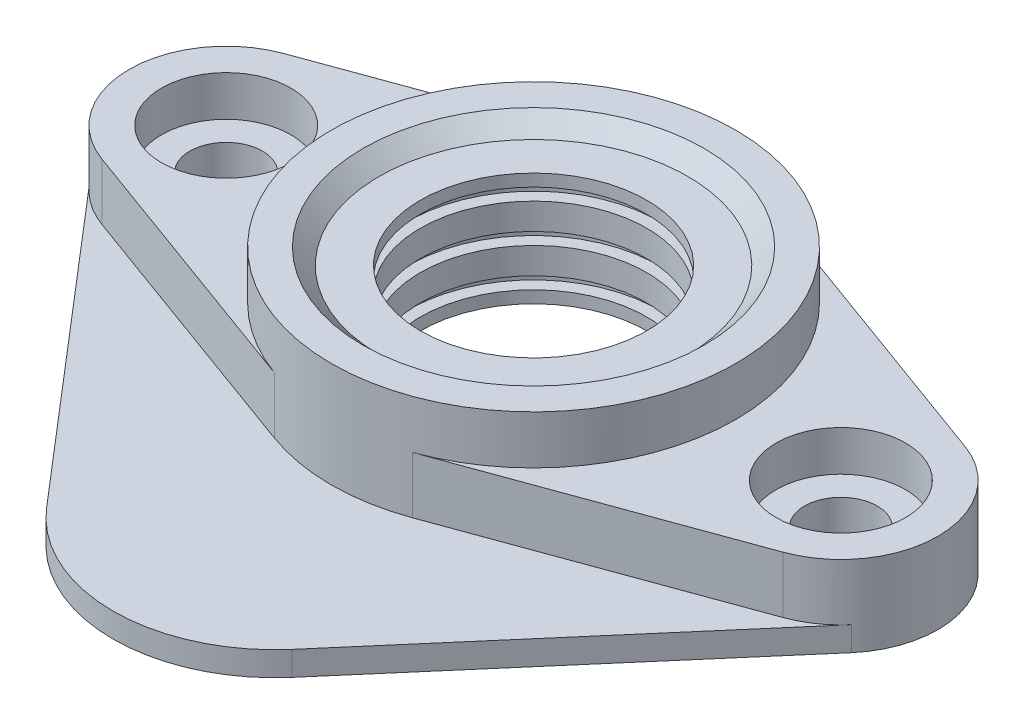
ISO-10303-21;
HEADER;
FILE_DESCRIPTION(('STEP AP214'),'2;1');
FILE_NAME('part.step','',(''),(''),'','','');
FILE_SCHEMA(('AUTOMOTIVE_DESIGN { 1 0 10303 214 1 1 1 1 }'));
ENDSEC;
DATA;
#1=APPLICATION_CONTEXT('core data for automotive mechanical design processes');
#2=APPLICATION_PROTOCOL_DEFINITION('international standard','automotive_design',2000,#1);
#3=PRODUCT_CONTEXT('',#1,'mechanical');
#4=PRODUCT('Part','Part','',(#3));
#5=PRODUCT_RELATED_PRODUCT_CATEGORY('part','',(#4));
#6=PRODUCT_DEFINITION_FORMATION('','',#4);
#7=PRODUCT_DEFINITION_CONTEXT('part definition',#1,'design');
#8=PRODUCT_DEFINITION('design','',#6,#7);
#9=PRODUCT_DEFINITION_SHAPE('','',#8);
#10=(LENGTH_UNIT() NAMED_UNIT(*) SI_UNIT(.MILLI.,.METRE.));
#11=(NAMED_UNIT(*) PLANE_ANGLE_UNIT() SI_UNIT($,.RADIAN.));
#12=(NAMED_UNIT(*) SI_UNIT($,.STERADIAN.) SOLID_ANGLE_UNIT());
#13=UNCERTAINTY_MEASURE_WITH_UNIT(LENGTH_MEASURE(1.E-05),#10,'distance_accuracy_value','');
#14=(GEOMETRIC_REPRESENTATION_CONTEXT(3) GLOBAL_UNCERTAINTY_ASSIGNED_CONTEXT((#13)) GLOBAL_UNIT_ASSIGNED_CONTEXT((#10,
#11,#12)) REPRESENTATION_CONTEXT('',''));
#15=CARTESIAN_POINT('',(0.,0.,0.));
#16=DIRECTION('',(0.,0.,1.));
#17=DIRECTION('',(1.,0.,0.));
#18=AXIS2_PLACEMENT_3D('',#15,#16,#17);
#19=CARTESIAN_POINT('',(-38.,3.,0.));
#20=DIRECTION('',(0.,1.,0.));
#21=DIRECTION('',(0.,0.,1.));
#22=AXIS2_PLACEMENT_3D('',#19,#20,#21);
#23=PLANE('',#22);
#24=DIRECTION('',(0.939661635334586,0.,-0.342105263157895));
#25=VECTOR('',#24,1.);
#26=CARTESIAN_POINT('',(8.55263157894737,3.,23.4915408833646));
#27=LINE('',#26,#25);
#28=CARTESIAN_POINT('',(8.55263157894736,3.,23.4915408833646));
#29=VERTEX_POINT('',#28);
#30=CARTESIAN_POINT('',(42.1052631578947,3.,11.275939624015));
#31=VERTEX_POINT('',#30);
#32=EDGE_CURVE('E69',#29,#31,#27,.T.);
#33=ORIENTED_EDGE('',*,*,#32,.F.);
#34=CARTESIAN_POINT('',(0.,3.,0.));
#35=DIRECTION('',(0.,1.,0.));
#36=DIRECTION('',(0.,0.,1.));
#37=AXIS2_PLACEMENT_3D('',#34,#35,#36);
#38=CIRCLE('',#37,25.);
#39=CARTESIAN_POINT('',(-8.55263157894736,3.,23.4915408833646));
#40=VERTEX_POINT('',#39);
#41=EDGE_CURVE('E264',#40,#29,#38,.T.);
#42=ORIENTED_EDGE('',*,*,#41,.F.);
#43=DIRECTION('',(0.939661635334586,0.,0.342105263157895));
#44=VECTOR('',#43,1.);
#45=CARTESIAN_POINT('',(-8.55263157894737,3.,23.4915408833646));
#46=LINE('',#45,#44);
#47=CARTESIAN_POINT('',(-42.1052631578947,3.,11.275939624015));
#48=VERTEX_POINT('',#47);
#49=EDGE_CURVE('E175',#48,#40,#46,.T.);
#50=ORIENTED_EDGE('',*,*,#49,.F.);
#51=CARTESIAN_POINT('',(-38.,3.,0.));
#52=DIRECTION('',(0.,1.,0.));
#53=DIRECTION('',(0.,0.,1.));
#54=AXIS2_PLACEMENT_3D('',#51,#52,#53);
#55=CIRCLE('',#54,12.);
#56=CARTESIAN_POINT('',(-47.1068684896246,3.,7.81440633142926));
#57=VERTEX_POINT('',#56);
#58=EDGE_CURVE('E11',#57,#48,#55,.T.);
#59=ORIENTED_EDGE('',*,*,#58,.F.);
#60=DIRECTION('',(0.651200527619105,0.,0.75890570746872));
#61=VECTOR('',#60,1.);
#62=CARTESIAN_POINT('',(-47.1068684896246,3.,7.81440633142926));
#63=LINE('',#62,#61);
#64=CARTESIAN_POINT('',(-15.1781141493744,3.,45.0240105523821));
#65=VERTEX_POINT('',#64);
#66=EDGE_CURVE('E192',#57,#65,#63,.T.);
#67=ORIENTED_EDGE('',*,*,#66,.T.);
#68=CARTESIAN_POINT('',(0.,3.,32.));
#69=DIRECTION('',(0.,1.,0.));
#70=DIRECTION('',(0.,0.,1.));
#71=AXIS2_PLACEMENT_3D('',#68,#69,#70);
#72=CIRCLE('',#71,20.);
#73=CARTESIAN_POINT('',(15.1781141493744,3.,45.0240105523821));
#74=VERTEX_POINT('',#73);
#75=EDGE_CURVE('E193',#65,#74,#72,.T.);
#76=ORIENTED_EDGE('',*,*,#75,.T.);
#77=DIRECTION('',(0.651200527619105,0.,-0.75890570746872));
#78=VECTOR('',#77,1.);
#79=CARTESIAN_POINT('',(47.1068684896246,3.,7.81440633142926));
#80=LINE('',#79,#78);
#81=CARTESIAN_POINT('',(47.1068684896246,3.,7.81440633142926));
#82=VERTEX_POINT('',#81);
#83=EDGE_CURVE('E197',#74,#82,#80,.T.);
#84=ORIENTED_EDGE('',*,*,#83,.T.);
#85=CARTESIAN_POINT('',(38.,3.,0.));
#86=DIRECTION('',(0.,1.,0.));
#87=DIRECTION('',(0.,0.,1.));
#88=AXIS2_PLACEMENT_3D('',#85,#86,#87);
#89=CIRCLE('',#88,12.);
#90=EDGE_CURVE('E61',#31,#82,#89,.T.);
#91=ORIENTED_EDGE('',*,*,#90,.F.);
#92=EDGE_LOOP('',(#33,#42,#50,#59,#67,#76,#84,#91));
#93=FACE_BOUND('',#92,.T.);
#94=ADVANCED_FACE('F50',(#93),#23,.T.);
#95=CARTESIAN_POINT('',(-38.,3.,0.));
#96=DIRECTION('',(0.,-1.,0.));
#97=DIRECTION('',(0.,0.,-1.));
#98=AXIS2_PLACEMENT_3D('',#95,#96,#97);
#99=CYLINDRICAL_SURFACE('',#98,12.);
#100=CARTESIAN_POINT('',(-38.,0.,0.));
#101=DIRECTION('',(0.,1.,0.));
#102=DIRECTION('',(0.,0.,1.));
#103=AXIS2_PLACEMENT_3D('',#100,#101,#102);
#104=CIRCLE('',#103,12.);
#105=CARTESIAN_POINT('',(-42.1052631578947,0.,-11.275939624015));
#106=VERTEX_POINT('',#105);
#107=CARTESIAN_POINT('',(-47.1068684896246,0.,7.81440633142926));
#108=VERTEX_POINT('',#107);
#109=EDGE_CURVE('E191',#106,#108,#104,.T.);
#110=ORIENTED_EDGE('',*,*,#109,.T.);
#111=DIRECTION('',(0.,-1.,0.));
#112=VECTOR('',#111,1.);
#113=CARTESIAN_POINT('',(-47.1068684896246,3.,7.81440633142926));
#114=LINE('',#113,#112);
#115=EDGE_CURVE('E51',#57,#108,#114,.T.);
#116=ORIENTED_EDGE('',*,*,#115,.F.);
#117=ORIENTED_EDGE('',*,*,#58,.T.);
#118=DIRECTION('',(0.,-1.,0.));
#119=VECTOR('',#118,1.);
#120=CARTESIAN_POINT('',(-42.1052631578947,10.,11.275939624015));
#121=LINE('',#120,#119);
#122=CARTESIAN_POINT('',(-42.1052631578947,10.,11.275939624015));
#123=VERTEX_POINT('',#122);
#124=EDGE_CURVE('E186',#123,#48,#121,.T.);
#125=ORIENTED_EDGE('',*,*,#124,.F.);
#126=CARTESIAN_POINT('',(-38.,10.,0.));
#127=DIRECTION('',(0.,1.,0.));
#128=DIRECTION('',(0.,0.,1.));
#129=AXIS2_PLACEMENT_3D('',#126,#127,#128);
#130=CIRCLE('',#129,12.);
#131=CARTESIAN_POINT('',(-42.1052631578947,10.,-11.275939624015));
#132=VERTEX_POINT('',#131);
#133=EDGE_CURVE('E176',#132,#123,#130,.T.);
#134=ORIENTED_EDGE('',*,*,#133,.F.);
#135=DIRECTION('',(0.,-1.,0.));
#136=VECTOR('',#135,1.);
#137=CARTESIAN_POINT('',(-42.1052631578947,3.,-11.275939624015));
#138=LINE('',#137,#136);
#139=EDGE_CURVE('E200',#132,#106,#138,.T.);
#140=ORIENTED_EDGE('',*,*,#139,.T.);
#141=EDGE_LOOP('',(#110,#116,#117,#125,#134,#140));
#142=FACE_BOUND('',#141,.T.);
#143=ADVANCED_FACE('F47',(#142),#99,.T.);
#144=CARTESIAN_POINT('',(-47.1068684896246,3.,7.81440633142926));
#145=DIRECTION('',(0.75890570746872,0.,-0.651200527619105));
#146=DIRECTION('',(-0.651200527619105,0.,-0.758905707468721));
#147=AXIS2_PLACEMENT_3D('',#144,#145,#146);
#148=PLANE('',#147);
#149=DIRECTION('',(0.651200527619105,0.,0.75890570746872));
#150=VECTOR('',#149,1.);
#151=CARTESIAN_POINT('',(-47.1068684896246,0.,7.81440633142926));
#152=LINE('',#151,#150);
#153=CARTESIAN_POINT('',(-15.1781141493744,0.,45.0240105523821));
#154=VERTEX_POINT('',#153);
#155=EDGE_CURVE('E205',#108,#154,#152,.T.);
#156=ORIENTED_EDGE('',*,*,#155,.T.);
#157=DIRECTION('',(0.,-1.,0.));
#158=VECTOR('',#157,1.);
#159=CARTESIAN_POINT('',(-15.1781141493744,3.,45.0240105523821));
#160=LINE('',#159,#158);
#161=EDGE_CURVE('E221',#65,#154,#160,.T.);
#162=ORIENTED_EDGE('',*,*,#161,.F.);
#163=ORIENTED_EDGE('',*,*,#66,.F.);
#164=ORIENTED_EDGE('',*,*,#115,.T.);
#165=EDGE_LOOP('',(#156,#162,#163,#164));
#166=FACE_BOUND('',#165,.T.);
#167=ADVANCED_FACE('F233',(#166),#148,.F.);
#168=CARTESIAN_POINT('',(0.,3.,32.));
#169=DIRECTION('',(0.,-1.,0.));
#170=DIRECTION('',(0.,0.,-1.));
#171=AXIS2_PLACEMENT_3D('',#168,#169,#170);
#172=CYLINDRICAL_SURFACE('',#171,20.);
#173=CARTESIAN_POINT('',(0.,0.,32.));
#174=DIRECTION('',(0.,1.,0.));
#175=DIRECTION('',(0.,0.,1.));
#176=AXIS2_PLACEMENT_3D('',#173,#174,#175);
#177=CIRCLE('',#176,20.);
#178=CARTESIAN_POINT('',(15.1781141493744,0.,45.0240105523821));
#179=VERTEX_POINT('',#178);
#180=EDGE_CURVE('E204',#154,#179,#177,.T.);
#181=ORIENTED_EDGE('',*,*,#180,.T.);
#182=DIRECTION('',(0.,-1.,0.));
#183=VECTOR('',#182,1.);
#184=CARTESIAN_POINT('',(15.1781141493744,3.,45.0240105523821));
#185=LINE('',#184,#183);
#186=EDGE_CURVE('E225',#74,#179,#185,.T.);
#187=ORIENTED_EDGE('',*,*,#186,.F.);
#188=ORIENTED_EDGE('',*,*,#75,.F.);
#189=ORIENTED_EDGE('',*,*,#161,.T.);
#190=EDGE_LOOP('',(#181,#187,#188,#189));
#191=FACE_BOUND('',#190,.T.);
#192=ADVANCED_FACE('F242',(#191),#172,.T.);
#193=CARTESIAN_POINT('',(47.1068684896246,3.,7.81440633142926));
#194=DIRECTION('',(-0.75890570746872,0.,-0.651200527619105));
#195=DIRECTION('',(-0.651200527619105,0.,0.758905707468721));
#196=AXIS2_PLACEMENT_3D('',#193,#194,#195);
#197=PLANE('',#196);
#198=DIRECTION('',(0.651200527619105,0.,-0.75890570746872));
#199=VECTOR('',#198,1.);
#200=CARTESIAN_POINT('',(47.1068684896246,0.,7.81440633142926));
#201=LINE('',#200,#199);
#202=CARTESIAN_POINT('',(47.1068684896246,0.,7.81440633142926));
#203=VERTEX_POINT('',#202);
#204=EDGE_CURVE('E206',#179,#203,#201,.T.);
#205=ORIENTED_EDGE('',*,*,#204,.T.);
#206=DIRECTION('',(0.,-1.,0.));
#207=VECTOR('',#206,1.);
#208=CARTESIAN_POINT('',(47.1068684896246,3.,7.81440633142926));
#209=LINE('',#208,#207);
#210=EDGE_CURVE('E218',#82,#203,#209,.T.);
#211=ORIENTED_EDGE('',*,*,#210,.F.);
#212=ORIENTED_EDGE('',*,*,#83,.F.);
#213=ORIENTED_EDGE('',*,*,#186,.T.);
#214=EDGE_LOOP('',(#205,#211,#212,#213));
#215=FACE_BOUND('',#214,.T.);
#216=ADVANCED_FACE('F247',(#215),#197,.F.);
#217=CARTESIAN_POINT('',(38.,3.,0.));
#218=DIRECTION('',(0.,-1.,0.));
#219=DIRECTION('',(0.,0.,-1.));
#220=AXIS2_PLACEMENT_3D('',#217,#218,#219);
#221=CYLINDRICAL_SURFACE('',#220,12.);
#222=CARTESIAN_POINT('',(38.,0.,0.));
#223=DIRECTION('',(0.,1.,0.));
#224=DIRECTION('',(0.,0.,1.));
#225=AXIS2_PLACEMENT_3D('',#222,#223,#224);
#226=CIRCLE('',#225,12.);
#227=CARTESIAN_POINT('',(42.1052631578947,0.,-11.275939624015));
#228=VERTEX_POINT('',#227);
#229=EDGE_CURVE('E208',#203,#228,#226,.T.);
#230=ORIENTED_EDGE('',*,*,#229,.T.);
#231=DIRECTION('',(0.,-1.,0.));
#232=VECTOR('',#231,1.);
#233=CARTESIAN_POINT('',(42.1052631578947,3.,-11.275939624015));
#234=LINE('',#233,#232);
#235=CARTESIAN_POINT('',(42.1052631578947,10.,-11.275939624015));
#236=VERTEX_POINT('',#235);
#237=EDGE_CURVE('E148',#236,#228,#234,.T.);
#238=ORIENTED_EDGE('',*,*,#237,.F.);
#239=CARTESIAN_POINT('',(38.,10.,0.));
#240=DIRECTION('',(0.,1.,0.));
#241=DIRECTION('',(0.,0.,1.));
#242=AXIS2_PLACEMENT_3D('',#239,#240,#241);
#243=CIRCLE('',#242,12.);
#244=CARTESIAN_POINT('',(42.1052631578947,10.,11.275939624015));
#245=VERTEX_POINT('',#244);
#246=EDGE_CURVE('E156',#245,#236,#243,.T.);
#247=ORIENTED_EDGE('',*,*,#246,.F.);
#248=DIRECTION('',(0.,-1.,0.));
#249=VECTOR('',#248,1.);
#250=CARTESIAN_POINT('',(42.1052631578947,10.,11.275939624015));
#251=LINE('',#250,#249);
#252=EDGE_CURVE('E162',#245,#31,#251,.T.);
#253=ORIENTED_EDGE('',*,*,#252,.T.);
#254=ORIENTED_EDGE('',*,*,#90,.T.);
#255=ORIENTED_EDGE('',*,*,#210,.T.);
#256=EDGE_LOOP('',(#230,#238,#247,#253,#254,#255));
#257=FACE_BOUND('',#256,.T.);
#258=ADVANCED_FACE('F261',(#257),#221,.T.);
#259=CARTESIAN_POINT('',(8.55263157894739,3.,-23.4915408833646));
#260=DIRECTION('',(-0.342105263157895,0.,0.939661635334585));
#261=DIRECTION('',(0.939661635334585,0.,0.342105263157895));
#262=AXIS2_PLACEMENT_3D('',#259,#260,#261);
#263=PLANE('',#262);
#264=DIRECTION('',(-0.939661635334585,0.,-0.342105263157895));
#265=VECTOR('',#264,1.);
#266=CARTESIAN_POINT('',(8.55263157894739,0.,-23.4915408833646));
#267=LINE('',#266,#265);
#268=CARTESIAN_POINT('',(8.55263157894739,0.,-23.4915408833646));
#269=VERTEX_POINT('',#268);
#270=EDGE_CURVE('E142',#228,#269,#267,.T.);
#271=ORIENTED_EDGE('',*,*,#270,.T.);
#272=DIRECTION('',(0.,-1.,0.));
#273=VECTOR('',#272,1.);
#274=CARTESIAN_POINT('',(8.55263157894739,3.,-23.4915408833646));
#275=LINE('',#274,#273);
#276=CARTESIAN_POINT('',(8.55263157894738,10.,-23.4915408833646));
#277=VERTEX_POINT('',#276);
#278=EDGE_CURVE('E136',#277,#269,#275,.T.);
#279=ORIENTED_EDGE('',*,*,#278,.F.);
#280=DIRECTION('',(-0.939661635334586,0.,-0.342105263157895));
#281=VECTOR('',#280,1.);
#282=CARTESIAN_POINT('',(8.55263157894738,10.,-23.4915408833646));
#283=LINE('',#282,#281);
#284=EDGE_CURVE('E140',#236,#277,#283,.T.);
#285=ORIENTED_EDGE('',*,*,#284,.F.);
#286=ORIENTED_EDGE('',*,*,#237,.T.);
#287=EDGE_LOOP('',(#271,#279,#285,#286));
#288=FACE_BOUND('',#287,.T.);
#289=ADVANCED_FACE('F139',(#288),#263,.F.);
#290=CARTESIAN_POINT('',(0.,3.,0.));
#291=DIRECTION('',(0.,-1.,0.));
#292=DIRECTION('',(0.,0.,-1.));
#293=AXIS2_PLACEMENT_3D('',#290,#291,#292);
#294=CYLINDRICAL_SURFACE('',#293,25.);
#295=CARTESIAN_POINT('',(0.,0.,0.));
#296=DIRECTION('',(0.,1.,0.));
#297=DIRECTION('',(0.,0.,1.));
#298=AXIS2_PLACEMENT_3D('',#295,#296,#297);
#299=CIRCLE('',#298,25.);
#300=CARTESIAN_POINT('',(-8.55263157894737,0.,-23.4915408833646));
#301=VERTEX_POINT('',#300);
#302=EDGE_CURVE('E211',#269,#301,#299,.T.);
#303=ORIENTED_EDGE('',*,*,#302,.T.);
#304=DIRECTION('',(0.,-1.,0.));
#305=VECTOR('',#304,1.);
#306=CARTESIAN_POINT('',(-8.55263157894737,3.,-23.4915408833646));
#307=LINE('',#306,#305);
#308=CARTESIAN_POINT('',(-8.55263157894737,10.,-23.4915408833646));
#309=VERTEX_POINT('',#308);
#310=EDGE_CURVE('E150',#309,#301,#307,.T.);
#311=ORIENTED_EDGE('',*,*,#310,.F.);
#312=CARTESIAN_POINT('',(0.,10.,0.));
#313=DIRECTION('',(0.,1.,0.));
#314=DIRECTION('',(0.,0.,1.));
#315=AXIS2_PLACEMENT_3D('',#312,#313,#314);
#316=CIRCLE('',#315,25.);
#317=CARTESIAN_POINT('',(-8.55263157894736,10.,23.4915408833646));
#318=VERTEX_POINT('',#317);
#319=EDGE_CURVE('E180',#309,#318,#316,.T.);
#320=ORIENTED_EDGE('',*,*,#319,.T.);
#321=DIRECTION('',(0.,-1.,0.));
#322=VECTOR('',#321,1.);
#323=CARTESIAN_POINT('',(-8.55263157894736,10.,23.4915408833646));
#324=LINE('',#323,#322);
#325=EDGE_CURVE('E185',#318,#40,#324,.T.);
#326=ORIENTED_EDGE('',*,*,#325,.T.);
#327=ORIENTED_EDGE('',*,*,#41,.T.);
#328=DIRECTION('',(0.,-1.,0.));
#329=VECTOR('',#328,1.);
#330=CARTESIAN_POINT('',(8.55263157894737,10.,23.4915408833646));
#331=LINE('',#330,#329);
#332=CARTESIAN_POINT('',(8.55263157894737,10.,23.4915408833646));
#333=VERTEX_POINT('',#332);
#334=EDGE_CURVE('E161',#333,#29,#331,.T.);
#335=ORIENTED_EDGE('',*,*,#334,.F.);
#336=CARTESIAN_POINT('',(0.,10.,0.));
#337=DIRECTION('',(0.,1.,0.));
#338=DIRECTION('',(0.,0.,1.));
#339=AXIS2_PLACEMENT_3D('',#336,#337,#338);
#340=CIRCLE('',#339,25.);
#341=EDGE_CURVE('E152',#333,#277,#340,.T.);
#342=ORIENTED_EDGE('',*,*,#341,.T.);
#343=ORIENTED_EDGE('',*,*,#278,.T.);
#344=EDGE_LOOP('',(#303,#311,#320,#326,#327,#335,#342,#343));
#345=FACE_BOUND('',#344,.T.);
#346=CARTESIAN_POINT('',(0.,16.,0.));
#347=DIRECTION('',(0.,1.,0.));
#348=DIRECTION('',(0.,0.,1.));
#349=AXIS2_PLACEMENT_3D('',#346,#347,#348);
#350=CIRCLE('',#349,25.);
#351=CARTESIAN_POINT('',(0.,16.,25.));
#352=VERTEX_POINT('',#351);
#353=EDGE_CURVE('E169',#352,#352,#350,.T.);
#354=ORIENTED_EDGE('',*,*,#353,.F.);
#355=EDGE_LOOP('',(#354));
#356=FACE_BOUND('',#355,.T.);
#357=ADVANCED_FACE('F158',(#345,#356),#294,.T.);
#358=CARTESIAN_POINT('',(-42.1052631578947,3.,-11.275939624015));
#359=DIRECTION('',(0.342105263157895,0.,0.939661635334585));
#360=DIRECTION('',(0.939661635334586,0.,-0.342105263157895));
#361=AXIS2_PLACEMENT_3D('',#358,#359,#360);
#362=PLANE('',#361);
#363=DIRECTION('',(-0.939661635334586,0.,0.342105263157895));
#364=VECTOR('',#363,1.);
#365=CARTESIAN_POINT('',(-42.1052631578947,0.,-11.275939624015));
#366=LINE('',#365,#364);
#367=EDGE_CURVE('E195',#301,#106,#366,.T.);
#368=ORIENTED_EDGE('',*,*,#367,.T.);
#369=ORIENTED_EDGE('',*,*,#139,.F.);
#370=DIRECTION('',(-0.939661635334586,0.,0.342105263157895));
#371=VECTOR('',#370,1.);
#372=CARTESIAN_POINT('',(-8.55263157894737,10.,-23.4915408833646));
#373=LINE('',#372,#371);
#374=EDGE_CURVE('E171',#309,#132,#373,.T.);
#375=ORIENTED_EDGE('',*,*,#374,.F.);
#376=ORIENTED_EDGE('',*,*,#310,.T.);
#377=EDGE_LOOP('',(#368,#369,#375,#376));
#378=FACE_BOUND('',#377,.T.);
#379=ADVANCED_FACE('F259',(#378),#362,.F.);
#380=CARTESIAN_POINT('',(-38.,0.,0.));
#381=DIRECTION('',(0.,1.,0.));
#382=DIRECTION('',(0.,0.,1.));
#383=AXIS2_PLACEMENT_3D('',#380,#381,#382);
#384=PLANE('',#383);
#385=CARTESIAN_POINT('',(38.,0.,0.));
#386=DIRECTION('',(0.,1.,0.));
#387=DIRECTION('',(0.,0.,1.));
#388=AXIS2_PLACEMENT_3D('',#385,#386,#387);
#389=CIRCLE('',#388,4.5);
#390=CARTESIAN_POINT('',(38.,0.,4.5));
#391=VERTEX_POINT('',#390);
#392=EDGE_CURVE('E322',#391,#391,#389,.T.);
#393=ORIENTED_EDGE('',*,*,#392,.T.);
#394=EDGE_LOOP('',(#393));
#395=FACE_BOUND('',#394,.T.);
#396=CARTESIAN_POINT('',(-38.,0.,0.));
#397=DIRECTION('',(0.,1.,0.));
#398=DIRECTION('',(0.,0.,1.));
#399=AXIS2_PLACEMENT_3D('',#396,#397,#398);
#400=CIRCLE('',#399,4.5);
#401=CARTESIAN_POINT('',(-38.,0.,4.5));
#402=VERTEX_POINT('',#401);
#403=EDGE_CURVE('E333',#402,#402,#400,.T.);
#404=ORIENTED_EDGE('',*,*,#403,.T.);
#405=EDGE_LOOP('',(#404));
#406=FACE_BOUND('',#405,.T.);
#407=CARTESIAN_POINT('',(0.,0.,0.));
#408=DIRECTION('',(0.,1.,0.));
#409=DIRECTION('',(0.,0.,1.));
#410=AXIS2_PLACEMENT_3D('',#407,#408,#409);
#411=CIRCLE('',#410,14.);
#412=CARTESIAN_POINT('',(0.,0.,14.));
#413=VERTEX_POINT('',#412);
#414=EDGE_CURVE('E271',#413,#413,#411,.T.);
#415=ORIENTED_EDGE('',*,*,#414,.T.);
#416=EDGE_LOOP('',(#415));
#417=FACE_BOUND('',#416,.T.);
#418=ORIENTED_EDGE('',*,*,#109,.F.);
#419=ORIENTED_EDGE('',*,*,#367,.F.);
#420=ORIENTED_EDGE('',*,*,#302,.F.);
#421=ORIENTED_EDGE('',*,*,#270,.F.);
#422=ORIENTED_EDGE('',*,*,#229,.F.);
#423=ORIENTED_EDGE('',*,*,#204,.F.);
#424=ORIENTED_EDGE('',*,*,#180,.F.);
#425=ORIENTED_EDGE('',*,*,#155,.F.);
#426=EDGE_LOOP('',(#418,#419,#420,#421,#422,#423,#424,#425));
#427=FACE_BOUND('',#426,.T.);
#428=ADVANCED_FACE('F238',(#395,#406,#417,#427),#384,.F.);
#429=CARTESIAN_POINT('',(-8.55263157894737,10.,23.4915408833646));
#430=DIRECTION('',(0.342105263157895,0.,-0.939661635334585));
#431=DIRECTION('',(-0.939661635334585,0.,-0.342105263157895));
#432=AXIS2_PLACEMENT_3D('',#429,#430,#431);
#433=PLANE('',#432);
#434=ORIENTED_EDGE('',*,*,#49,.T.);
#435=ORIENTED_EDGE('',*,*,#325,.F.);
#436=DIRECTION('',(0.939661635334586,0.,0.342105263157895));
#437=VECTOR('',#436,1.);
#438=CARTESIAN_POINT('',(-8.55263157894737,10.,23.4915408833646));
#439=LINE('',#438,#437);
#440=EDGE_CURVE('E179',#123,#318,#439,.T.);
#441=ORIENTED_EDGE('',*,*,#440,.F.);
#442=ORIENTED_EDGE('',*,*,#124,.T.);
#443=EDGE_LOOP('',(#434,#435,#441,#442));
#444=FACE_BOUND('',#443,.T.);
#445=ADVANCED_FACE('F252',(#444),#433,.F.);
#446=CARTESIAN_POINT('',(0.,10.,0.));
#447=DIRECTION('',(0.,1.,0.));
#448=DIRECTION('',(0.,0.,1.));
#449=AXIS2_PLACEMENT_3D('',#446,#447,#448);
#450=PLANE('',#449);
#451=CARTESIAN_POINT('',(-38.,10.,0.));
#452=DIRECTION('',(0.,1.,0.));
#453=DIRECTION('',(0.,0.,1.));
#454=AXIS2_PLACEMENT_3D('',#451,#452,#453);
#455=CIRCLE('',#454,8.);
#456=CARTESIAN_POINT('',(-38.,10.,8.));
#457=VERTEX_POINT('',#456);
#458=EDGE_CURVE('E319',#457,#457,#455,.T.);
#459=ORIENTED_EDGE('',*,*,#458,.F.);
#460=EDGE_LOOP('',(#459));
#461=FACE_BOUND('',#460,.T.);
#462=ORIENTED_EDGE('',*,*,#374,.T.);
#463=ORIENTED_EDGE('',*,*,#133,.T.);
#464=ORIENTED_EDGE('',*,*,#440,.T.);
#465=ORIENTED_EDGE('',*,*,#319,.F.);
#466=EDGE_LOOP('',(#462,#463,#464,#465));
#467=FACE_BOUND('',#466,.T.);
#468=ADVANCED_FACE('F258',(#461,#467),#450,.T.);
#469=CARTESIAN_POINT('',(8.55263157894737,10.,23.4915408833646));
#470=DIRECTION('',(-0.342105263157895,0.,-0.939661635334585));
#471=DIRECTION('',(-0.939661635334586,0.,0.342105263157895));
#472=AXIS2_PLACEMENT_3D('',#469,#470,#471);
#473=PLANE('',#472);
#474=ORIENTED_EDGE('',*,*,#32,.T.);
#475=ORIENTED_EDGE('',*,*,#252,.F.);
#476=DIRECTION('',(0.939661635334586,0.,-0.342105263157895));
#477=VECTOR('',#476,1.);
#478=CARTESIAN_POINT('',(8.55263157894737,10.,23.4915408833646));
#479=LINE('',#478,#477);
#480=EDGE_CURVE('E166',#333,#245,#479,.T.);
#481=ORIENTED_EDGE('',*,*,#480,.F.);
#482=ORIENTED_EDGE('',*,*,#334,.T.);
#483=EDGE_LOOP('',(#474,#475,#481,#482));
#484=FACE_BOUND('',#483,.T.);
#485=ADVANCED_FACE('F262',(#484),#473,.F.);
#486=CARTESIAN_POINT('',(0.,10.,0.));
#487=DIRECTION('',(0.,1.,0.));
#488=DIRECTION('',(0.,0.,1.));
#489=AXIS2_PLACEMENT_3D('',#486,#487,#488);
#490=PLANE('',#489);
#491=CARTESIAN_POINT('',(38.,10.,0.));
#492=DIRECTION('',(0.,1.,0.));
#493=DIRECTION('',(0.,0.,1.));
#494=AXIS2_PLACEMENT_3D('',#491,#492,#493);
#495=CIRCLE('',#494,8.);
#496=CARTESIAN_POINT('',(38.,10.,8.));
#497=VERTEX_POINT('',#496);
#498=EDGE_CURVE('E330',#497,#497,#495,.T.);
#499=ORIENTED_EDGE('',*,*,#498,.F.);
#500=EDGE_LOOP('',(#499));
#501=FACE_BOUND('',#500,.T.);
#502=ORIENTED_EDGE('',*,*,#480,.T.);
#503=ORIENTED_EDGE('',*,*,#246,.T.);
#504=ORIENTED_EDGE('',*,*,#284,.T.);
#505=ORIENTED_EDGE('',*,*,#341,.F.);
#506=EDGE_LOOP('',(#502,#503,#504,#505));
#507=FACE_BOUND('',#506,.T.);
#508=ADVANCED_FACE('F153',(#501,#507),#490,.T.);
#509=CARTESIAN_POINT('',(0.,16.,0.));
#510=DIRECTION('',(0.,1.,0.));
#511=DIRECTION('',(0.,0.,1.));
#512=AXIS2_PLACEMENT_3D('',#509,#510,#511);
#513=PLANE('',#512);
#514=CARTESIAN_POINT('',(0.,16.,0.));
#515=DIRECTION('',(0.,1.,0.));
#516=DIRECTION('',(0.,0.,1.));
#517=AXIS2_PLACEMENT_3D('',#514,#515,#516);
#518=CIRCLE('',#517,21.0839676538374);
#519=CARTESIAN_POINT('',(0.,16.,21.0839676538374));
#520=VERTEX_POINT('',#519);
#521=EDGE_CURVE('E266',#520,#520,#518,.T.);
#522=ORIENTED_EDGE('',*,*,#521,.F.);
#523=EDGE_LOOP('',(#522));
#524=FACE_BOUND('',#523,.T.);
#525=ORIENTED_EDGE('',*,*,#353,.T.);
#526=EDGE_LOOP('',(#525));
#527=FACE_BOUND('',#526,.T.);
#528=ADVANCED_FACE('F366',(#524,#527),#513,.T.);
#529=CARTESIAN_POINT('',(0.,14.,0.));
#530=DIRECTION('',(0.,1.,0.));
#531=DIRECTION('',(0.,0.,1.));
#532=AXIS2_PLACEMENT_3D('',#529,#530,#531);
#533=CONICAL_SURFACE('',#532,19.0839676538374,0.785398163397447);
#534=ORIENTED_EDGE('',*,*,#521,.T.);
#535=EDGE_LOOP('',(#534));
#536=FACE_BOUND('',#535,.T.);
#537=CARTESIAN_POINT('',(0.,14.,0.));
#538=DIRECTION('',(0.,1.,0.));
#539=DIRECTION('',(0.,0.,1.));
#540=AXIS2_PLACEMENT_3D('',#537,#538,#539);
#541=CIRCLE('',#540,19.0839676538374);
#542=CARTESIAN_POINT('',(0.,14.,19.0839676538374));
#543=VERTEX_POINT('',#542);
#544=EDGE_CURVE('E316',#543,#543,#541,.T.);
#545=ORIENTED_EDGE('',*,*,#544,.F.);
#546=EDGE_LOOP('',(#545));
#547=FACE_BOUND('',#546,.T.);
#548=ADVANCED_FACE('F372',(#536,#547),#533,.F.);
#549=CARTESIAN_POINT('',(0.,16.,0.));
#550=DIRECTION('',(0.,1.,0.));
#551=DIRECTION('',(0.,0.,1.));
#552=AXIS2_PLACEMENT_3D('',#549,#550,#551);
#553=CYLINDRICAL_SURFACE('',#552,14.);
#554=CARTESIAN_POINT('',(0.,1.5,0.));
#555=DIRECTION('',(0.,1.,0.));
#556=DIRECTION('',(0.,0.,1.));
#557=AXIS2_PLACEMENT_3D('',#554,#555,#556);
#558=CIRCLE('',#557,14.);
#559=CARTESIAN_POINT('',(0.,1.5,14.));
#560=VERTEX_POINT('',#559);
#561=EDGE_CURVE('E280',#560,#560,#558,.T.);
#562=ORIENTED_EDGE('',*,*,#561,.T.);
#563=EDGE_LOOP('',(#562));
#564=FACE_BOUND('',#563,.T.);
#565=ORIENTED_EDGE('',*,*,#414,.F.);
#566=EDGE_LOOP('',(#565));
#567=FACE_BOUND('',#566,.T.);
#568=ADVANCED_FACE('F467',(#564,#567),#553,.F.);
#569=CARTESIAN_POINT('',(15.5,1.5,0.));
#570=DIRECTION('',(0.,1.,0.));
#571=DIRECTION('',(0.,0.,1.));
#572=AXIS2_PLACEMENT_3D('',#569,#570,#571);
#573=PLANE('',#572);
#574=CARTESIAN_POINT('',(0.,1.5,0.));
#575=DIRECTION('',(0.,1.,0.));
#576=DIRECTION('',(0.,0.,1.));
#577=AXIS2_PLACEMENT_3D('',#574,#575,#576);
#578=CIRCLE('',#577,15.5);
#579=CARTESIAN_POINT('',(0.,1.5,15.5));
#580=VERTEX_POINT('',#579);
#581=EDGE_CURVE('E278',#580,#580,#578,.T.);
#582=ORIENTED_EDGE('',*,*,#581,.T.);
#583=EDGE_LOOP('',(#582));
#584=FACE_BOUND('',#583,.T.);
#585=ORIENTED_EDGE('',*,*,#561,.F.);
#586=EDGE_LOOP('',(#585));
#587=FACE_BOUND('',#586,.T.);
#588=ADVANCED_FACE('F478',(#584,#587),#573,.T.);
#589=CARTESIAN_POINT('',(0.,16.,0.));
#590=DIRECTION('',(0.,1.,0.));
#591=DIRECTION('',(0.,0.,1.));
#592=AXIS2_PLACEMENT_3D('',#589,#590,#591);
#593=CYLINDRICAL_SURFACE('',#592,15.5);
#594=CARTESIAN_POINT('',(0.,3.,0.));
#595=DIRECTION('',(0.,1.,0.));
#596=DIRECTION('',(0.,0.,1.));
#597=AXIS2_PLACEMENT_3D('',#594,#595,#596);
#598=CIRCLE('',#597,15.5);
#599=CARTESIAN_POINT('',(0.,3.,15.5));
#600=VERTEX_POINT('',#599);
#601=EDGE_CURVE('E281',#600,#600,#598,.T.);
#602=ORIENTED_EDGE('',*,*,#601,.T.);
#603=EDGE_LOOP('',(#602));
#604=FACE_BOUND('',#603,.T.);
#605=ORIENTED_EDGE('',*,*,#581,.F.);
#606=EDGE_LOOP('',(#605));
#607=FACE_BOUND('',#606,.T.);
#608=ADVANCED_FACE('F484',(#604,#607),#593,.F.);
#609=CARTESIAN_POINT('',(14.,3.,0.));
#610=DIRECTION('',(0.,-1.,0.));
#611=DIRECTION('',(0.,0.,-1.));
#612=AXIS2_PLACEMENT_3D('',#609,#610,#611);
#613=PLANE('',#612);
#614=CARTESIAN_POINT('',(0.,3.,0.));
#615=DIRECTION('',(0.,1.,0.));
#616=DIRECTION('',(0.,0.,1.));
#617=AXIS2_PLACEMENT_3D('',#614,#615,#616);
#618=CIRCLE('',#617,14.);
#619=CARTESIAN_POINT('',(0.,3.,14.));
#620=VERTEX_POINT('',#619);
#621=EDGE_CURVE('E286',#620,#620,#618,.T.);
#622=ORIENTED_EDGE('',*,*,#621,.T.);
#623=EDGE_LOOP('',(#622));
#624=FACE_BOUND('',#623,.T.);
#625=ORIENTED_EDGE('',*,*,#601,.F.);
#626=EDGE_LOOP('',(#625));
#627=FACE_BOUND('',#626,.T.);
#628=ADVANCED_FACE('F493',(#624,#627),#613,.T.);
#629=CARTESIAN_POINT('',(0.,16.,0.));
#630=DIRECTION('',(0.,1.,0.));
#631=DIRECTION('',(0.,0.,1.));
#632=AXIS2_PLACEMENT_3D('',#629,#630,#631);
#633=CYLINDRICAL_SURFACE('',#632,14.);
#634=CARTESIAN_POINT('',(0.,6.25,0.));
#635=DIRECTION('',(0.,1.,0.));
#636=DIRECTION('',(0.,0.,1.));
#637=AXIS2_PLACEMENT_3D('',#634,#635,#636);
#638=CIRCLE('',#637,14.);
#639=CARTESIAN_POINT('',(0.,6.25,14.));
#640=VERTEX_POINT('',#639);
#641=EDGE_CURVE('E288',#640,#640,#638,.T.);
#642=ORIENTED_EDGE('',*,*,#641,.T.);
#643=EDGE_LOOP('',(#642));
#644=FACE_BOUND('',#643,.T.);
#645=ORIENTED_EDGE('',*,*,#621,.F.);
#646=EDGE_LOOP('',(#645));
#647=FACE_BOUND('',#646,.T.);
#648=ADVANCED_FACE('F501',(#644,#647),#633,.F.);
#649=CARTESIAN_POINT('',(15.5,6.25,0.));
#650=DIRECTION('',(0.,1.,0.));
#651=DIRECTION('',(0.,0.,1.));
#652=AXIS2_PLACEMENT_3D('',#649,#650,#651);
#653=PLANE('',#652);
#654=CARTESIAN_POINT('',(0.,6.25,0.));
#655=DIRECTION('',(0.,1.,0.));
#656=DIRECTION('',(0.,0.,1.));
#657=AXIS2_PLACEMENT_3D('',#654,#655,#656);
#658=CIRCLE('',#657,15.5);
#659=CARTESIAN_POINT('',(0.,6.25,15.5));
#660=VERTEX_POINT('',#659);
#661=EDGE_CURVE('E295',#660,#660,#658,.T.);
#662=ORIENTED_EDGE('',*,*,#661,.T.);
#663=EDGE_LOOP('',(#662));
#664=FACE_BOUND('',#663,.T.);
#665=ORIENTED_EDGE('',*,*,#641,.F.);
#666=EDGE_LOOP('',(#665));
#667=FACE_BOUND('',#666,.T.);
#668=ADVANCED_FACE('F515',(#664,#667),#653,.T.);
#669=CARTESIAN_POINT('',(0.,16.,0.));
#670=DIRECTION('',(0.,1.,0.));
#671=DIRECTION('',(0.,0.,1.));
#672=AXIS2_PLACEMENT_3D('',#669,#670,#671);
#673=CYLINDRICAL_SURFACE('',#672,15.5);
#674=CARTESIAN_POINT('',(0.,7.75,0.));
#675=DIRECTION('',(0.,1.,0.));
#676=DIRECTION('',(0.,0.,1.));
#677=AXIS2_PLACEMENT_3D('',#674,#675,#676);
#678=CIRCLE('',#677,15.5);
#679=CARTESIAN_POINT('',(0.,7.75,15.5));
#680=VERTEX_POINT('',#679);
#681=EDGE_CURVE('E293',#680,#680,#678,.T.);
#682=ORIENTED_EDGE('',*,*,#681,.T.);
#683=EDGE_LOOP('',(#682));
#684=FACE_BOUND('',#683,.T.);
#685=ORIENTED_EDGE('',*,*,#661,.F.);
#686=EDGE_LOOP('',(#685));
#687=FACE_BOUND('',#686,.T.);
#688=ADVANCED_FACE('F521',(#684,#687),#673,.F.);
#689=CARTESIAN_POINT('',(14.,7.75,0.));
#690=DIRECTION('',(0.,-1.,0.));
#691=DIRECTION('',(0.,0.,-1.));
#692=AXIS2_PLACEMENT_3D('',#689,#690,#691);
#693=PLANE('',#692);
#694=CARTESIAN_POINT('',(0.,7.75,0.));
#695=DIRECTION('',(0.,1.,0.));
#696=DIRECTION('',(0.,0.,1.));
#697=AXIS2_PLACEMENT_3D('',#694,#695,#696);
#698=CIRCLE('',#697,14.);
#699=CARTESIAN_POINT('',(0.,7.75,14.));
#700=VERTEX_POINT('',#699);
#701=EDGE_CURVE('E296',#700,#700,#698,.T.);
#702=ORIENTED_EDGE('',*,*,#701,.T.);
#703=EDGE_LOOP('',(#702));
#704=FACE_BOUND('',#703,.T.);
#705=ORIENTED_EDGE('',*,*,#681,.F.);
#706=EDGE_LOOP('',(#705));
#707=FACE_BOUND('',#706,.T.);
#708=ADVANCED_FACE('F529',(#704,#707),#693,.T.);
#709=CARTESIAN_POINT('',(0.,16.,0.));
#710=DIRECTION('',(0.,1.,0.));
#711=DIRECTION('',(0.,0.,1.));
#712=AXIS2_PLACEMENT_3D('',#709,#710,#711);
#713=CYLINDRICAL_SURFACE('',#712,14.);
#714=CARTESIAN_POINT('',(0.,11.,0.));
#715=DIRECTION('',(0.,1.,0.));
#716=DIRECTION('',(0.,0.,1.));
#717=AXIS2_PLACEMENT_3D('',#714,#715,#716);
#718=CIRCLE('',#717,14.);
#719=CARTESIAN_POINT('',(0.,11.,14.));
#720=VERTEX_POINT('',#719);
#721=EDGE_CURVE('E301',#720,#720,#718,.T.);
#722=ORIENTED_EDGE('',*,*,#721,.T.);
#723=EDGE_LOOP('',(#722));
#724=FACE_BOUND('',#723,.T.);
#725=ORIENTED_EDGE('',*,*,#701,.F.);
#726=EDGE_LOOP('',(#725));
#727=FACE_BOUND('',#726,.T.);
#728=ADVANCED_FACE('F537',(#724,#727),#713,.F.);
#729=CARTESIAN_POINT('',(15.5,11.,0.));
#730=DIRECTION('',(0.,1.,0.));
#731=DIRECTION('',(0.,0.,1.));
#732=AXIS2_PLACEMENT_3D('',#729,#730,#731);
#733=PLANE('',#732);
#734=CARTESIAN_POINT('',(0.,11.,0.));
#735=DIRECTION('',(0.,1.,0.));
#736=DIRECTION('',(0.,0.,1.));
#737=AXIS2_PLACEMENT_3D('',#734,#735,#736);
#738=CIRCLE('',#737,15.5);
#739=CARTESIAN_POINT('',(0.,11.,15.5));
#740=VERTEX_POINT('',#739);
#741=EDGE_CURVE('E303',#740,#740,#738,.T.);
#742=ORIENTED_EDGE('',*,*,#741,.T.);
#743=EDGE_LOOP('',(#742));
#744=FACE_BOUND('',#743,.T.);
#745=ORIENTED_EDGE('',*,*,#721,.F.);
#746=EDGE_LOOP('',(#745));
#747=FACE_BOUND('',#746,.T.);
#748=ADVANCED_FACE('F547',(#744,#747),#733,.T.);
#749=CARTESIAN_POINT('',(0.,16.,0.));
#750=DIRECTION('',(0.,1.,0.));
#751=DIRECTION('',(0.,0.,1.));
#752=AXIS2_PLACEMENT_3D('',#749,#750,#751);
#753=CYLINDRICAL_SURFACE('',#752,15.5);
#754=CARTESIAN_POINT('',(0.,12.5,0.));
#755=DIRECTION('',(0.,1.,0.));
#756=DIRECTION('',(0.,0.,1.));
#757=AXIS2_PLACEMENT_3D('',#754,#755,#756);
#758=CIRCLE('',#757,15.5);
#759=CARTESIAN_POINT('',(0.,12.5,15.5));
#760=VERTEX_POINT('',#759);
#761=EDGE_CURVE('E307',#760,#760,#758,.T.);
#762=ORIENTED_EDGE('',*,*,#761,.T.);
#763=EDGE_LOOP('',(#762));
#764=FACE_BOUND('',#763,.T.);
#765=ORIENTED_EDGE('',*,*,#741,.F.);
#766=EDGE_LOOP('',(#765));
#767=FACE_BOUND('',#766,.T.);
#768=ADVANCED_FACE('F560',(#764,#767),#753,.F.);
#769=CARTESIAN_POINT('',(14.,12.5,0.));
#770=DIRECTION('',(0.,-1.,0.));
#771=DIRECTION('',(0.,0.,-1.));
#772=AXIS2_PLACEMENT_3D('',#769,#770,#771);
#773=PLANE('',#772);
#774=CARTESIAN_POINT('',(0.,12.5,0.));
#775=DIRECTION('',(0.,1.,0.));
#776=DIRECTION('',(0.,0.,1.));
#777=AXIS2_PLACEMENT_3D('',#774,#775,#776);
#778=CIRCLE('',#777,14.);
#779=CARTESIAN_POINT('',(0.,12.5,14.));
#780=VERTEX_POINT('',#779);
#781=EDGE_CURVE('E309',#780,#780,#778,.T.);
#782=ORIENTED_EDGE('',*,*,#781,.T.);
#783=EDGE_LOOP('',(#782));
#784=FACE_BOUND('',#783,.T.);
#785=ORIENTED_EDGE('',*,*,#761,.F.);
#786=EDGE_LOOP('',(#785));
#787=FACE_BOUND('',#786,.T.);
#788=ADVANCED_FACE('F567',(#784,#787),#773,.T.);
#789=CARTESIAN_POINT('',(0.,16.,0.));
#790=DIRECTION('',(0.,1.,0.));
#791=DIRECTION('',(0.,0.,1.));
#792=AXIS2_PLACEMENT_3D('',#789,#790,#791);
#793=CYLINDRICAL_SURFACE('',#792,14.);
#794=CARTESIAN_POINT('',(0.,14.,0.));
#795=DIRECTION('',(0.,1.,0.));
#796=DIRECTION('',(0.,0.,1.));
#797=AXIS2_PLACEMENT_3D('',#794,#795,#796);
#798=CIRCLE('',#797,14.);
#799=CARTESIAN_POINT('',(0.,14.,14.));
#800=VERTEX_POINT('',#799);
#801=EDGE_CURVE('E311',#800,#800,#798,.T.);
#802=ORIENTED_EDGE('',*,*,#801,.T.);
#803=EDGE_LOOP('',(#802));
#804=FACE_BOUND('',#803,.T.);
#805=ORIENTED_EDGE('',*,*,#781,.F.);
#806=EDGE_LOOP('',(#805));
#807=FACE_BOUND('',#806,.T.);
#808=ADVANCED_FACE('F574',(#804,#807),#793,.F.);
#809=CARTESIAN_POINT('',(14.,14.,0.));
#810=DIRECTION('',(0.,1.,0.));
#811=DIRECTION('',(0.,0.,1.));
#812=AXIS2_PLACEMENT_3D('',#809,#810,#811);
#813=PLANE('',#812);
#814=ORIENTED_EDGE('',*,*,#544,.T.);
#815=EDGE_LOOP('',(#814));
#816=FACE_BOUND('',#815,.T.);
#817=ORIENTED_EDGE('',*,*,#801,.F.);
#818=EDGE_LOOP('',(#817));
#819=FACE_BOUND('',#818,.T.);
#820=ADVANCED_FACE('F361',(#816,#819),#813,.T.);
#821=CARTESIAN_POINT('',(38.,5.,0.));
#822=DIRECTION('',(0.,1.,0.));
#823=DIRECTION('',(0.,0.,1.));
#824=AXIS2_PLACEMENT_3D('',#821,#822,#823);
#825=CYLINDRICAL_SURFACE('',#824,8.);
#826=CARTESIAN_POINT('',(38.,5.,0.));
#827=DIRECTION('',(0.,1.,0.));
#828=DIRECTION('',(0.,0.,1.));
#829=AXIS2_PLACEMENT_3D('',#826,#827,#828);
#830=CIRCLE('',#829,8.);
#831=CARTESIAN_POINT('',(38.,5.,8.));
#832=VERTEX_POINT('',#831);
#833=EDGE_CURVE('E317',#832,#832,#830,.T.);
#834=ORIENTED_EDGE('',*,*,#833,.F.);
#835=EDGE_LOOP('',(#834));
#836=FACE_BOUND('',#835,.T.);
#837=ORIENTED_EDGE('',*,*,#498,.T.);
#838=EDGE_LOOP('',(#837));
#839=FACE_BOUND('',#838,.T.);
#840=ADVANCED_FACE('F357',(#836,#839),#825,.F.);
#841=CARTESIAN_POINT('',(38.,5.,0.));
#842=DIRECTION('',(0.,1.,0.));
#843=DIRECTION('',(0.,0.,1.));
#844=AXIS2_PLACEMENT_3D('',#841,#842,#843);
#845=PLANE('',#844);
#846=CARTESIAN_POINT('',(38.,5.,0.));
#847=DIRECTION('',(0.,1.,0.));
#848=DIRECTION('',(0.,0.,1.));
#849=AXIS2_PLACEMENT_3D('',#846,#847,#848);
#850=CIRCLE('',#849,4.5);
#851=CARTESIAN_POINT('',(38.,5.,4.5));
#852=VERTEX_POINT('',#851);
#853=EDGE_CURVE('E336',#852,#852,#850,.T.);
#854=ORIENTED_EDGE('',*,*,#853,.F.);
#855=EDGE_LOOP('',(#854));
#856=FACE_BOUND('',#855,.T.);
#857=ORIENTED_EDGE('',*,*,#833,.T.);
#858=EDGE_LOOP('',(#857));
#859=FACE_BOUND('',#858,.T.);
#860=ADVANCED_FACE('F351',(#856,#859),#845,.T.);
#861=CARTESIAN_POINT('',(-38.,5.,0.));
#862=DIRECTION('',(0.,1.,0.));
#863=DIRECTION('',(0.,0.,1.));
#864=AXIS2_PLACEMENT_3D('',#861,#862,#863);
#865=CYLINDRICAL_SURFACE('',#864,8.);
#866=CARTESIAN_POINT('',(-38.,5.,0.));
#867=DIRECTION('',(0.,1.,0.));
#868=DIRECTION('',(0.,0.,1.));
#869=AXIS2_PLACEMENT_3D('',#866,#867,#868);
#870=CIRCLE('',#869,8.);
#871=CARTESIAN_POINT('',(-38.,5.,8.));
#872=VERTEX_POINT('',#871);
#873=EDGE_CURVE('E323',#872,#872,#870,.T.);
#874=ORIENTED_EDGE('',*,*,#873,.F.);
#875=EDGE_LOOP('',(#874));
#876=FACE_BOUND('',#875,.T.);
#877=ORIENTED_EDGE('',*,*,#458,.T.);
#878=EDGE_LOOP('',(#877));
#879=FACE_BOUND('',#878,.T.);
#880=ADVANCED_FACE('F356',(#876,#879),#865,.F.);
#881=CARTESIAN_POINT('',(-38.,5.,0.));
#882=DIRECTION('',(0.,1.,0.));
#883=DIRECTION('',(0.,0.,1.));
#884=AXIS2_PLACEMENT_3D('',#881,#882,#883);
#885=PLANE('',#884);
#886=CARTESIAN_POINT('',(-38.,5.,0.));
#887=DIRECTION('',(0.,1.,0.));
#888=DIRECTION('',(0.,0.,1.));
#889=AXIS2_PLACEMENT_3D('',#886,#887,#888);
#890=CIRCLE('',#889,4.5);
#891=CARTESIAN_POINT('',(-38.,5.,4.5));
#892=VERTEX_POINT('',#891);
#893=EDGE_CURVE('E335',#892,#892,#890,.T.);
#894=ORIENTED_EDGE('',*,*,#893,.F.);
#895=EDGE_LOOP('',(#894));
#896=FACE_BOUND('',#895,.T.);
#897=ORIENTED_EDGE('',*,*,#873,.T.);
#898=EDGE_LOOP('',(#897));
#899=FACE_BOUND('',#898,.T.);
#900=ADVANCED_FACE('F616',(#896,#899),#885,.T.);
#901=CARTESIAN_POINT('',(-38.,0.,0.));
#902=DIRECTION('',(0.,1.,0.));
#903=DIRECTION('',(0.,0.,1.));
#904=AXIS2_PLACEMENT_3D('',#901,#902,#903);
#905=CYLINDRICAL_SURFACE('',#904,4.5);
#906=ORIENTED_EDGE('',*,*,#403,.F.);
#907=EDGE_LOOP('',(#906));
#908=FACE_BOUND('',#907,.T.);
#909=ORIENTED_EDGE('',*,*,#893,.T.);
#910=EDGE_LOOP('',(#909));
#911=FACE_BOUND('',#910,.T.);
#912=ADVANCED_FACE('F349',(#908,#911),#905,.F.);
#913=CARTESIAN_POINT('',(38.,0.,0.));
#914=DIRECTION('',(0.,1.,0.));
#915=DIRECTION('',(0.,0.,1.));
#916=AXIS2_PLACEMENT_3D('',#913,#914,#915);
#917=CYLINDRICAL_SURFACE('',#916,4.5);
#918=ORIENTED_EDGE('',*,*,#392,.F.);
#919=EDGE_LOOP('',(#918));
#920=FACE_BOUND('',#919,.T.);
#921=ORIENTED_EDGE('',*,*,#853,.T.);
#922=EDGE_LOOP('',(#921));
#923=FACE_BOUND('',#922,.T.);
#924=ADVANCED_FACE('F347',(#920,#923),#917,.F.);
#925=CLOSED_SHELL('',(#94,#143,#167,#192,#216,#258,#289,#357,#379,#428,#445,#468,#485,#508,#528,
#548,#568,#588,#608,#628,#648,#668,#688,#708,#728,#748,#768,#788,#808,#820,#840,#860,#880,#900,
#912,#924));
#926=MANIFOLD_SOLID_BREP('B2',#925);
#927=ADVANCED_BREP_SHAPE_REPRESENTATION('',(#18,#926),#14);
#928=SHAPE_DEFINITION_REPRESENTATION(#9,#927);
ENDSEC;
END-ISO-10303-21;
